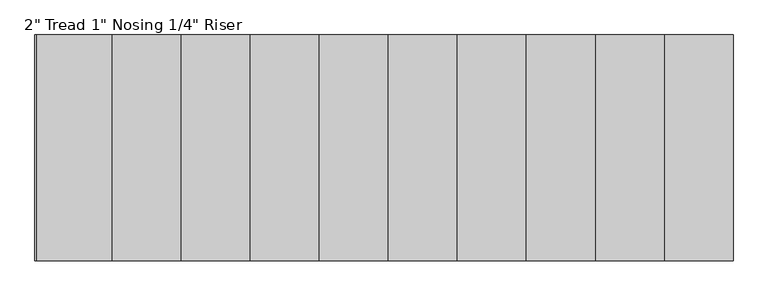
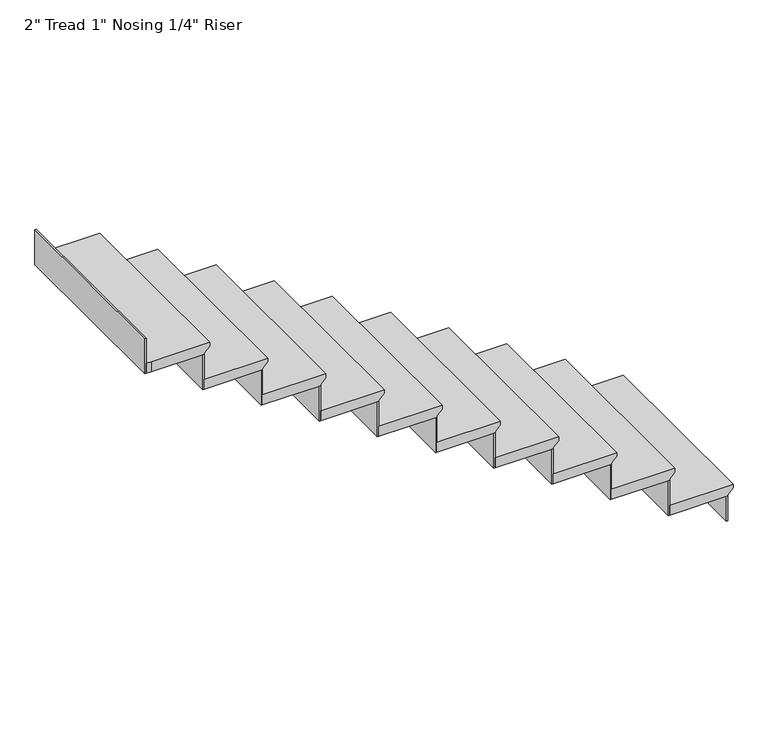
"""IFC4 building model written with IfcOpenShell, lengths in millimetres: stair flight geometry."""

from ifc_helpers import new_model, si_unit, origin, place, context, project, spatial, faceted_brep, source, transform, mapped, element, save


def stair_flight_c6e2231d(model_context):
    return source(origin(), model_context, "Body", "Brep", [
        faceted_brep([(23001.1136801, 4885.2409313, 768.35), (23001.1136801, 4885.2409313, 787.4), (23001.1136801, 3970.8409313, 787.4), (23001.1136801, 3970.8409313, 768.35), (22975.7136801, 4885.2409313, 742.95), (22975.7136801, 3970.8409313, 742.95), (22696.3136801, 4885.2409313, 787.4), (22696.3136801, 3970.8409313, 787.4), (22975.7136801, 3970.8409313, 736.6), (22696.3136801, 3970.8409313, 736.6), (22696.3136801, 4885.2409313, 736.6), (22975.7136801, 4885.2409313, 736.6)], [[[0, 1, 2, 3]], [[4, 0, 3, 5]], [[2, 1, 6, 7]], [[8, 9, 10, 11]], [[2, 7, 9, 8, 5, 3]], [[8, 11, 4, 5]], [[6, 1, 0, 4, 11, 10]], [[7, 6, 10, 9]]]),
        faceted_brep([(22975.7136801, 4885.2409313, 736.6), (22975.7136801, 4885.2409313, 609.6), (22969.3636801, 4885.2409313, 609.6), (22969.3636801, 4885.2409313, 736.6), (22975.7136801, 3970.8409313, 736.6), (22969.3636801, 3970.8409313, 736.6), (22969.3636801, 3970.8409313, 609.6), (22975.7136801, 3970.8409313, 609.6)], [[[0, 1, 2, 3]], [[4, 5, 6, 7]], [[1, 0, 4, 7]], [[2, 1, 7, 6]], [[3, 2, 6, 5]], [[0, 3, 5, 4]]]),
        faceted_brep([(22696.3136801, 4885.2409313, 914.4), (22696.3136801, 4885.2409313, 736.6), (22689.9636801, 4885.2409313, 736.6), (22689.9636801, 4885.2409313, 914.4), (22696.3136801, 3970.8409313, 914.4), (22689.9636801, 3970.8409313, 914.4), (22689.9636801, 3970.8409313, 736.6), (22696.3136801, 3970.8409313, 736.6)], [[[0, 1, 2, 3]], [[4, 5, 6, 7]], [[1, 0, 4, 7]], [[2, 1, 7, 6]], [[3, 2, 6, 5]], [[0, 3, 5, 4]]]),
        faceted_brep([(22721.7136801, 3970.8409313, 965.2), (22721.7136801, 4885.2409313, 965.2), (22416.9136801, 4885.2409313, 965.2), (22416.9136801, 3970.8409313, 965.2), (22696.3136801, 3970.8409313, 914.4), (22416.9136801, 3970.8409313, 914.4), (22416.9136801, 4885.2409313, 914.4), (22696.3136801, 4885.2409313, 914.4), (22696.3136801, 3970.8409313, 920.75), (22721.7136801, 3970.8409313, 946.15), (22696.3136801, 4885.2409313, 920.75), (22721.7136801, 4885.2409313, 946.15)], [[[0, 1, 2, 3]], [[4, 5, 6, 7]], [[0, 3, 5, 4, 8, 9]], [[4, 7, 10, 8]], [[2, 1, 11, 10, 7, 6]], [[3, 2, 6, 5]], [[11, 1, 0, 9]], [[10, 11, 9, 8]]]),
        faceted_brep([(22416.9136801, 4885.2409313, 1092.2), (22416.9136801, 4885.2409313, 914.4), (22410.5636801, 4885.2409313, 914.4), (22410.5636801, 4885.2409313, 1092.2), (22416.9136801, 3970.8409313, 1092.2), (22410.5636801, 3970.8409313, 1092.2), (22410.5636801, 3970.8409313, 914.4), (22416.9136801, 3970.8409313, 914.4)], [[[0, 1, 2, 3]], [[4, 5, 6, 7]], [[1, 0, 4, 7]], [[2, 1, 7, 6]], [[3, 2, 6, 5]], [[0, 3, 5, 4]]]),
        faceted_brep([(22442.3136801, 3970.8409313, 1143.0), (22442.3136801, 4885.2409313, 1143.0), (22137.5136801, 4885.2409313, 1143.0), (22137.5136801, 3970.8409313, 1143.0), (22416.9136801, 3970.8409313, 1092.2), (22137.5136801, 3970.8409313, 1092.2), (22137.5136801, 4885.2409313, 1092.2), (22416.9136801, 4885.2409313, 1092.2), (22416.9136801, 3970.8409313, 1098.55), (22442.3136801, 3970.8409313, 1123.95), (22416.9136801, 4885.2409313, 1098.55), (22442.3136801, 4885.2409313, 1123.95)], [[[0, 1, 2, 3]], [[4, 5, 6, 7]], [[0, 3, 5, 4, 8, 9]], [[4, 7, 10, 8]], [[2, 1, 11, 10, 7, 6]], [[3, 2, 6, 5]], [[11, 1, 0, 9]], [[10, 11, 9, 8]]]),
        faceted_brep([(22137.5136801, 4885.2409313, 1270.0), (22137.5136801, 4885.2409313, 1092.2), (22131.1636801, 4885.2409313, 1092.2), (22131.1636801, 4885.2409313, 1270.0), (22137.5136801, 3970.8409313, 1270.0), (22131.1636801, 3970.8409313, 1270.0), (22131.1636801, 3970.8409313, 1092.2), (22137.5136801, 3970.8409313, 1092.2)], [[[0, 1, 2, 3]], [[4, 5, 6, 7]], [[1, 0, 4, 7]], [[2, 1, 7, 6]], [[3, 2, 6, 5]], [[0, 3, 5, 4]]]),
        faceted_brep([(22162.9136801, 3970.8409313, 1320.8), (22162.9136801, 4885.2409313, 1320.8), (21858.1136801, 4885.2409313, 1320.8), (21858.1136801, 3970.8409313, 1320.8), (22137.5136801, 3970.8409313, 1270.0), (21858.1136801, 3970.8409313, 1270.0), (21858.1136801, 4885.2409313, 1270.0), (22137.5136801, 4885.2409313, 1270.0), (22137.5136801, 3970.8409313, 1276.35), (22162.9136801, 3970.8409313, 1301.75), (22137.5136801, 4885.2409313, 1276.35), (22162.9136801, 4885.2409313, 1301.75)], [[[0, 1, 2, 3]], [[4, 5, 6, 7]], [[0, 3, 5, 4, 8, 9]], [[4, 7, 10, 8]], [[2, 1, 11, 10, 7, 6]], [[3, 2, 6, 5]], [[11, 1, 0, 9]], [[10, 11, 9, 8]]]),
        faceted_brep([(21858.1136801, 4885.2409313, 1447.8), (21858.1136801, 4885.2409313, 1270.0), (21851.7636801, 4885.2409313, 1270.0), (21851.7636801, 4885.2409313, 1447.8), (21858.1136801, 3970.8409313, 1447.8), (21851.7636801, 3970.8409313, 1447.8), (21851.7636801, 3970.8409313, 1270.0), (21858.1136801, 3970.8409313, 1270.0)], [[[0, 1, 2, 3]], [[4, 5, 6, 7]], [[1, 0, 4, 7]], [[2, 1, 7, 6]], [[3, 2, 6, 5]], [[0, 3, 5, 4]]]),
        faceted_brep([(21883.5136801, 3970.8409313, 1498.6), (21883.5136801, 4885.2409313, 1498.6), (21578.7136801, 4885.2409313, 1498.6), (21578.7136801, 3970.8409313, 1498.6), (21858.1136801, 3970.8409313, 1447.8), (21578.7136801, 3970.8409313, 1447.8), (21578.7136801, 4885.2409313, 1447.8), (21858.1136801, 4885.2409313, 1447.8), (21858.1136801, 3970.8409313, 1454.15), (21883.5136801, 3970.8409313, 1479.55), (21858.1136801, 4885.2409313, 1454.15), (21883.5136801, 4885.2409313, 1479.55)], [[[0, 1, 2, 3]], [[4, 5, 6, 7]], [[0, 3, 5, 4, 8, 9]], [[4, 7, 10, 8]], [[2, 1, 11, 10, 7, 6]], [[3, 2, 6, 5]], [[11, 1, 0, 9]], [[10, 11, 9, 8]]]),
        faceted_brep([(21578.7136801, 4885.2409313, 1625.6), (21578.7136801, 4885.2409313, 1447.8), (21572.3636801, 4885.2409313, 1447.8), (21572.3636801, 4885.2409313, 1625.6), (21578.7136801, 3970.8409313, 1625.6), (21572.3636801, 3970.8409313, 1625.6), (21572.3636801, 3970.8409313, 1447.8), (21578.7136801, 3970.8409313, 1447.8)], [[[0, 1, 2, 3]], [[4, 5, 6, 7]], [[1, 0, 4, 7]], [[2, 1, 7, 6]], [[3, 2, 6, 5]], [[0, 3, 5, 4]]]),
        faceted_brep([(21604.1136801, 3970.8409313, 1676.4), (21604.1136801, 4885.2409313, 1676.4), (21299.3136801, 4885.2409313, 1676.4), (21299.3136801, 3970.8409313, 1676.4), (21578.7136801, 3970.8409313, 1625.6), (21299.3136801, 3970.8409313, 1625.6), (21299.3136801, 4885.2409313, 1625.6), (21578.7136801, 4885.2409313, 1625.6), (21578.7136801, 3970.8409313, 1631.95), (21604.1136801, 3970.8409313, 1657.35), (21578.7136801, 4885.2409313, 1631.95), (21604.1136801, 4885.2409313, 1657.35)], [[[0, 1, 2, 3]], [[4, 5, 6, 7]], [[0, 3, 5, 4, 8, 9]], [[4, 7, 10, 8]], [[2, 1, 11, 10, 7, 6]], [[3, 2, 6, 5]], [[11, 1, 0, 9]], [[10, 11, 9, 8]]]),
        faceted_brep([(21299.3136801, 4885.2409313, 1803.4), (21299.3136801, 4885.2409313, 1625.6), (21292.9636801, 4885.2409313, 1625.6), (21292.9636801, 4885.2409313, 1803.4), (21299.3136801, 3970.8409313, 1803.4), (21292.9636801, 3970.8409313, 1803.4), (21292.9636801, 3970.8409313, 1625.6), (21299.3136801, 3970.8409313, 1625.6)], [[[0, 1, 2, 3]], [[4, 5, 6, 7]], [[1, 0, 4, 7]], [[2, 1, 7, 6]], [[3, 2, 6, 5]], [[0, 3, 5, 4]]]),
        faceted_brep([(21324.7136801, 3970.8409313, 1854.2), (21324.7136801, 4885.2409313, 1854.2), (21019.9136801, 4885.2409313, 1854.2), (21019.9136801, 3970.8409313, 1854.2), (21299.3136801, 3970.8409313, 1803.4), (21019.9136801, 3970.8409313, 1803.4), (21019.9136801, 4885.2409313, 1803.4), (21299.3136801, 4885.2409313, 1803.4), (21299.3136801, 3970.8409313, 1809.75), (21324.7136801, 3970.8409313, 1835.15), (21299.3136801, 4885.2409313, 1809.75), (21324.7136801, 4885.2409313, 1835.15)], [[[0, 1, 2, 3]], [[4, 5, 6, 7]], [[0, 3, 5, 4, 8, 9]], [[4, 7, 10, 8]], [[2, 1, 11, 10, 7, 6]], [[3, 2, 6, 5]], [[11, 1, 0, 9]], [[10, 11, 9, 8]]]),
        faceted_brep([(21019.9136801, 4885.2409313, 1981.2), (21019.9136801, 4885.2409313, 1803.4), (21013.5636801, 4885.2409313, 1803.4), (21013.5636801, 4885.2409313, 1981.2), (21019.9136801, 3970.8409313, 1981.2), (21013.5636801, 3970.8409313, 1981.2), (21013.5636801, 3970.8409313, 1803.4), (21019.9136801, 3970.8409313, 1803.4)], [[[0, 1, 2, 3]], [[4, 5, 6, 7]], [[1, 0, 4, 7]], [[2, 1, 7, 6]], [[3, 2, 6, 5]], [[0, 3, 5, 4]]]),
        faceted_brep([(21045.3136801, 3970.8409313, 2032.0), (21045.3136801, 4885.2409313, 2032.0), (20740.5136801, 4885.2409313, 2032.0), (20740.5136801, 3970.8409313, 2032.0), (21019.9136801, 3970.8409313, 1981.2), (20740.5136801, 3970.8409313, 1981.2), (20740.5136801, 4885.2409313, 1981.2), (21019.9136801, 4885.2409313, 1981.2), (21019.9136801, 3970.8409313, 1987.55), (21045.3136801, 3970.8409313, 2012.95), (21019.9136801, 4885.2409313, 1987.55), (21045.3136801, 4885.2409313, 2012.95)], [[[0, 1, 2, 3]], [[4, 5, 6, 7]], [[0, 3, 5, 4, 8, 9]], [[4, 7, 10, 8]], [[2, 1, 11, 10, 7, 6]], [[3, 2, 6, 5]], [[11, 1, 0, 9]], [[10, 11, 9, 8]]]),
        faceted_brep([(20740.5136801, 4885.2409313, 2159.0), (20740.5136801, 4885.2409313, 1981.2), (20734.1636801, 4885.2409313, 1981.2), (20734.1636801, 4885.2409313, 2159.0), (20740.5136801, 3970.8409313, 2159.0), (20734.1636801, 3970.8409313, 2159.0), (20734.1636801, 3970.8409313, 1981.2), (20740.5136801, 3970.8409313, 1981.2)], [[[0, 1, 2, 3]], [[4, 5, 6, 7]], [[1, 0, 4, 7]], [[2, 1, 7, 6]], [[3, 2, 6, 5]], [[0, 3, 5, 4]]]),
        faceted_brep([(20765.9136801, 3970.8409313, 2209.8), (20765.9136801, 4885.2409313, 2209.8), (20461.1136801, 4885.2409313, 2209.8), (20461.1136801, 3970.8409313, 2209.8), (20740.5136801, 3970.8409313, 2159.0), (20461.1136801, 3970.8409313, 2159.0), (20461.1136801, 4885.2409313, 2159.0), (20740.5136801, 4885.2409313, 2159.0), (20740.5136801, 3970.8409313, 2165.35), (20765.9136801, 3970.8409313, 2190.75), (20740.5136801, 4885.2409313, 2165.35), (20765.9136801, 4885.2409313, 2190.75)], [[[0, 1, 2, 3]], [[4, 5, 6, 7]], [[0, 3, 5, 4, 8, 9]], [[4, 7, 10, 8]], [[2, 1, 11, 10, 7, 6]], [[3, 2, 6, 5]], [[11, 1, 0, 9]], [[10, 11, 9, 8]]]),
        faceted_brep([(20181.7136801, 4885.2409313, 2514.6), (20181.7136801, 4885.2409313, 2336.8), (20175.3636801, 4885.2409313, 2336.8), (20175.3636801, 4885.2409313, 2514.6), (20181.7136801, 3970.8409313, 2514.6), (20175.3636801, 3970.8409313, 2514.6), (20175.3636801, 3970.8409313, 2336.8), (20181.7136801, 3970.8409313, 2336.8)], [[[0, 1, 2, 3]], [[4, 5, 6, 7]], [[1, 0, 4, 7]], [[2, 1, 7, 6]], [[3, 2, 6, 5]], [[0, 3, 5, 4]]]),
        faceted_brep([(20461.1136801, 4885.2409313, 2336.8), (20461.1136801, 4885.2409313, 2159.0), (20454.7636801, 4885.2409313, 2159.0), (20454.7636801, 4885.2409313, 2336.8), (20461.1136801, 3970.8409313, 2336.8), (20454.7636801, 3970.8409313, 2336.8), (20454.7636801, 3970.8409313, 2159.0), (20461.1136801, 3970.8409313, 2159.0)], [[[0, 1, 2, 3]], [[4, 5, 6, 7]], [[1, 0, 4, 7]], [[2, 1, 7, 6]], [[3, 2, 6, 5]], [[0, 3, 5, 4]]]),
        faceted_brep([(20181.7136801, 3970.8409313, 2387.6), (20207.1136801, 3970.8409313, 2387.6), (20486.5136801, 3970.8409313, 2387.6), (20486.5136801, 4885.2409313, 2387.6), (20181.7136801, 4885.2409313, 2387.6), (20207.1136801, 3970.8409313, 2336.8), (20181.7136801, 3970.8409313, 2336.8), (20181.7136801, 4885.2409313, 2336.8), (20461.1136801, 4885.2409313, 2336.8), (20461.1136801, 3970.8409313, 2336.8), (20461.1136801, 3970.8409313, 2343.15), (20486.5136801, 3970.8409313, 2368.55), (20461.1136801, 4885.2409313, 2343.15), (20486.5136801, 4885.2409313, 2368.55)], [[[0, 1, 2, 3, 4]], [[5, 6, 7, 8, 9]], [[1, 0, 6, 5]], [[2, 1, 5, 9, 10, 11]], [[9, 8, 12, 10]], [[4, 3, 13, 12, 8, 7]], [[0, 4, 7, 6]], [[13, 3, 2, 11]], [[12, 13, 11, 10]]]),
    ])


if __name__ == "__main__":
    model = new_model("IFC4")
    model_context = context("Model", 3, world=origin())
    ifc_project = project(units=[si_unit("LENGTHUNIT", "METRE", prefix="MILLI")], contexts=[model_context])
    site = spatial("IfcSite", under=ifc_project)
    building = spatial("IfcBuilding", under=site)
    placement = place(None, origin())
    stair_flight_shape = stair_flight_c6e2231d(model_context)
    element("IfcStairFlight", 1, ObjectType="2\" Tread 1\" Nosing 1/4\" Riser", at=placement, inside=building, context=model_context, shape_type="MappedRepresentation", body=[
        mapped(stair_flight_shape, transform((0.0, 0.0, 0.0), x_axis=(1.0, 0.0, 0.0), y_axis=(0.0, 1.0, 0.0), z_axis=(0.0, 0.0, 1.0))),
    ])
    save(model, "model.ifc")
